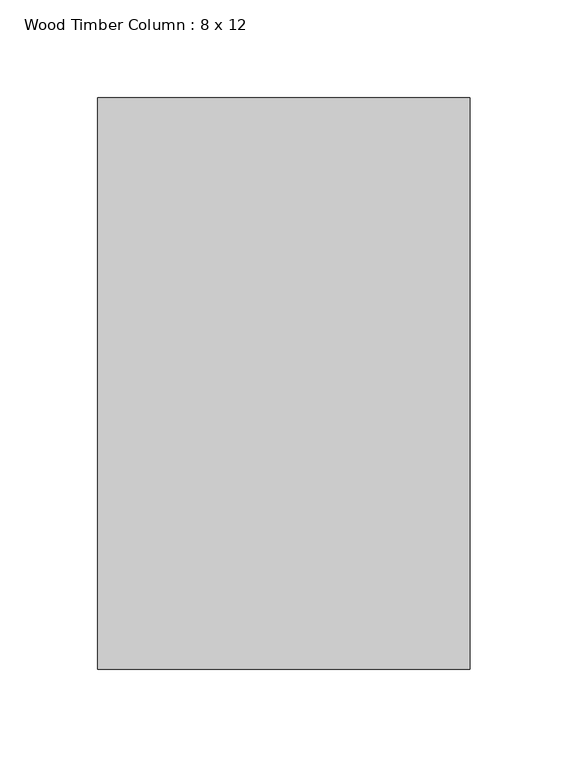
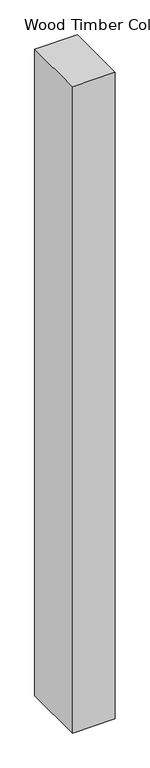
"""IFC4 building model written with IfcOpenShell, lengths in millimetres: column geometry, Wood Timber Column : 8 x 12."""

from ifc_helpers import new_model, si_unit, frame, origin, place, context, project, spatial, polyline, outline, extrude, source, transform, mapped, element, save


def wood_timber_column_8_x_12_4a74a8f5(model_context):
    return source(origin(), model_context, "Body", "SweptSolid", [
        extrude(outline(polyline([(95.25, -146.05), (-95.25, -146.05), (-95.25, 146.05), (95.25, 146.05), (95.25, -146.05)])), frame((0.0, 0.0, 3946.3794859), z_axis=(0.0, 0.0, 1.0), x_axis=(1.0, 0.0, 0.0)), (0.0, 0.0, 1.0), 3048.0),
    ])


if __name__ == "__main__":
    model = new_model("IFC4")
    model_context = context("Model", 3, world=origin())
    ifc_project = project(units=[si_unit("LENGTHUNIT", "METRE", prefix="MILLI")], contexts=[model_context])
    site = spatial("IfcSite", under=ifc_project)
    building = spatial("IfcBuilding", under=site)
    placement = place(None, origin())
    wood_timber_column_8_x_12_shape = wood_timber_column_8_x_12_4a74a8f5(model_context)
    element("IfcColumn", 1, ObjectType="Wood Timber Column : 8 x 12", at=placement, inside=building, context=model_context, shape_type="MappedRepresentation", body=[
        mapped(wood_timber_column_8_x_12_shape, transform((0.0, 0.0, 0.0), x_axis=(1.0, 0.0, 0.0), y_axis=(0.0, 1.0, 0.0), z_axis=(0.0, 0.0, 1.0))),
    ])
    save(model, "model.ifc")

# Revit data of these elements
# Type "Wood Timber Column : 8 x 12"
#   Assembly Code = "B1010200"
#   Depth = 0' - 11 1/2"
#   Width = 0' - 7 1/2"
#   Material = Softwood, Lumber
# Element 1 (IfcColumn, "Wood Timber Column : 8 x 12")
#   Materials on its faces: "Softwood, Lumber"
# Materials
#   "Softwood, Lumber": class "Wood", colour RGB 223 192 134, transparency 0, Description = "Pinus Echinata", Cost = 0
